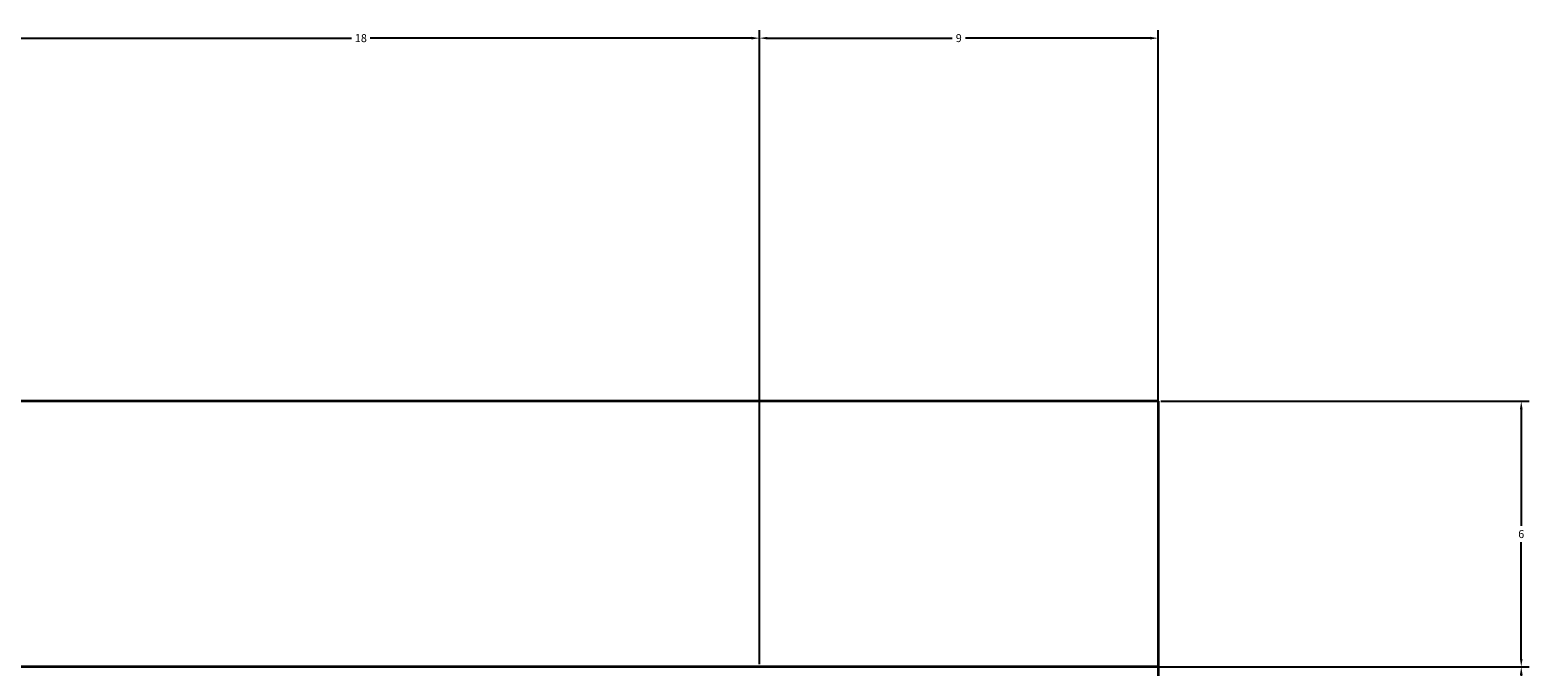
# Model space of a CAD drawing. Units: inches. Extents: x 27 to 200, y -50 to 102.
# Tile 26 of 26: x 166 to 200, y 88 to 102. Entities that reach past the tile are written whole.
import ezdxf

# ---------------------------------------------------------------- set-up
doc = ezdxf.new("R2010")
doc.units = ezdxf.units.IN
doc.header["$MEASUREMENT"] = 0
doc.layers.add('A-ANNO-DIMS', color=2, linetype='Continuous', lineweight=18)
doc.layers.add('A-ELEV', color=7, linetype='Continuous', lineweight=35)
doc.styles.get("Standard").update_dxf_attribs({"font": 'arial.ttf'})
doc.dimstyles.get("Standard").update_dxf_attribs({"dimtxt": 0.18, "dimasz": 0.18, "dimexe": 0.18, "dimexo": 0.0625, "dimgap": 0.09, "dimtad": 0, "dimtih": 1, "dimtoh": 1, "dimdec": 4, "dimzin": 0, "dimdsep": 46, "dimtxsty": 'Standard', "dimcen": 0.09, "dimadec": 0, "dimazin": 0, "dimtfac": 1, "dimtdec": 4, "dimtofl": 0, "dimtmove": 0, "dimatfit": 3, "dimfxl": 1, "dimtolj": 1, "dimtzin": 0, "dimarcsym": 0})

# ---------------------------------------------------------------- blocks, each defined once
blk = doc.blocks.new('*D21')
at = {"layer": 'A-ANNO-DIMS', "color": 0, "lineweight": -2, "transparency": 16777216}
for p, q in [((164.417, 87.989), (164.417, 102.306)), ((164.597, 102.126), (173.206, 102.126)), ((182.237, 102.126), (173.628, 102.126)), ((182.417, 87.989), (182.417, 102.306))]:
    blk.add_line(p, q, dxfattribs=at)
at = {"layer": 'A-ANNO-DIMS', "color": 0, "transparency": 16777216}
for points in [[(164.597, 102.156), (164.597, 102.096), (164.417, 102.126)], [(182.237, 102.156), (182.237, 102.096), (182.417, 102.126)]]:
    blk.add_solid(points, dxfattribs=at)
at = {"layer": 'Defpoints', "color": 0, "transparency": 16777216}
for p in [(182.417, 102.126), (164.417, 87.926), (182.417, 87.926)]:
    blk.add_point(p, dxfattribs=at)
at = {"layer": 'A-ANNO-DIMS', "color": 0, "transparency": 16777216, "insert": (173.417, 102.126), "char_height": 0.18, "attachment_point": 5}
blk.add_mtext('\\A1;18', dxfattribs=at)
blk = doc.blocks.new('*D22')
at = {"layer": 'A-ANNO-DIMS', "color": 0, "lineweight": -2, "transparency": 16777216}
for p, q in [((182.417, 87.989), (182.417, 102.306)), ((182.597, 102.126), (186.768, 102.126)), ((191.237, 102.126), (187.066, 102.126)), ((191.417, 87.989), (191.417, 102.306))]:
    blk.add_line(p, q, dxfattribs=at)
at = {"layer": 'A-ANNO-DIMS', "color": 0, "transparency": 16777216}
for points in [[(182.597, 102.156), (182.597, 102.096), (182.417, 102.126)], [(191.237, 102.156), (191.237, 102.096), (191.417, 102.126)]]:
    blk.add_solid(points, dxfattribs=at)
at = {"layer": 'Defpoints', "color": 0, "transparency": 16777216}
for p in [(191.417, 102.126), (182.417, 87.926), (191.417, 87.926)]:
    blk.add_point(p, dxfattribs=at)
at = {"layer": 'A-ANNO-DIMS', "color": 0, "transparency": 16777216, "insert": (186.917, 102.126), "char_height": 0.18, "attachment_point": 5}
blk.add_mtext('\\A1;9', dxfattribs=at)
blk = doc.blocks.new('*D31')
at = {"layer": 'A-ANNO-DIMS', "color": 0, "lineweight": -2, "transparency": 16777216}
for p, q in [((146.479, 87.926), (199.797, 87.926)), ((199.617, 87.746), (199.617, 77.845)), ((199.617, 67.579), (199.617, 77.481)), ((146.479, 67.399), (199.797, 67.399))]:
    blk.add_line(p, q, dxfattribs=at)
at = {"layer": 'A-ANNO-DIMS', "color": 0, "transparency": 16777216}
for points in [[(199.587, 87.746), (199.647, 87.746), (199.617, 87.926)], [(199.587, 67.579), (199.647, 67.579), (199.617, 67.399)]]:
    blk.add_solid(points, dxfattribs=at)
at = {"layer": 'Defpoints', "color": 0, "transparency": 16777216}
for p in [(146.417, 87.926), (199.617, 87.926), (146.417, 67.399)]:
    blk.add_point(p, dxfattribs=at)
at = {"layer": 'A-ANNO-DIMS', "color": 0, "transparency": 16777216, "insert": (199.617, 77.663), "char_height": 0.18, "attachment_point": 5}
blk.add_mtext('\\A1;20.527', dxfattribs=at)
blk = doc.blocks.new('*D32')
at = {"layer": 'A-ANNO-DIMS', "color": 0, "lineweight": -2, "transparency": 16777216}
for p, q in [((191.479, 93.926), (199.797, 93.926)), ((199.617, 93.746), (199.617, 91.108)), ((199.617, 88.106), (199.617, 90.745)), ((191.479, 87.926), (199.797, 87.926))]:
    blk.add_line(p, q, dxfattribs=at)
at = {"layer": 'A-ANNO-DIMS', "color": 0, "transparency": 16777216}
for points in [[(199.587, 93.746), (199.647, 93.746), (199.617, 93.926)], [(199.587, 88.106), (199.647, 88.106), (199.617, 87.926)]]:
    blk.add_solid(points, dxfattribs=at)
at = {"layer": 'Defpoints', "color": 0, "transparency": 16777216}
for p in [(191.417, 93.926), (199.617, 93.926), (191.417, 87.926)]:
    blk.add_point(p, dxfattribs=at)
at = {"layer": 'A-ANNO-DIMS', "color": 0, "transparency": 16777216, "insert": (199.617, 90.926), "char_height": 0.18, "attachment_point": 5}
blk.add_mtext('\\A1;6', dxfattribs=at)

msp = doc.modelspace()

# ---------------------------------------------------------------- linework, layer by layer
at = {"layer": 'A-ELEV'}
for p, q in [((191.4169, 93.9264), (35.4169, 93.9264)), ((191.4169, 93.9264), (191.4169, -16.7693)), ((191.4169, 87.9264), (35.4169, 87.9264))]:
    msp.add_line(p, q, dxfattribs=at)

# ---------------------------------------------------------------- dimensions: what is measured, and where the dimension line sits
at = {"layer": 'A-ANNO-DIMS'}
for base, p1, p2, picture, middle in [((182.4169, 102.1264), (164.4169, 87.9264), (182.4169, 87.9264), '*D21', (173.4169, 102.1264)), ((191.4169, 102.1264), (182.4169, 87.9264), (191.4169, 87.9264), '*D22', (186.9169, 102.1264))]:
    dim = msp.add_linear_dim(base=base, p1=p1, p2=p2, dimstyle='Standard', override={"dimdec": 0, "dimlfac": 1, "dimrnd": 0, "dimzin": 0, "dimdsep": 46, "dimlunit": 2}, dxfattribs=at)
    dim.commit()
    dim.dimension.update_dxf_attribs({"geometry": picture, "text_midpoint": middle})
for base, p1, p2, override, picture, middle in [((199.6169, 93.9264), (191.4169, 87.9264), (191.4169, 93.9264), {"dimdec": 0, "dimlfac": 1, "dimrnd": 0, "dimzin": 0, "dimdsep": 46, "dimlunit": 2}, '*D32', (199.6169, 90.9264)), ((199.6169, 87.9264), (146.4169, 67.3991), (146.4169, 87.9264), {"dimdec": 3, "dimlfac": 1, "dimrnd": 0, "dimzin": 0, "dimdsep": 46, "dimlunit": 2}, '*D31', (199.6169, 77.6628))]:
    dim = msp.add_linear_dim(base=base, p1=p1, p2=p2, angle=90, dimstyle='Standard', override=override, dxfattribs=at)
    dim.commit()
    dim.dimension.update_dxf_attribs({"geometry": picture, "text_midpoint": middle})

doc.saveas('drawing.dxf')
